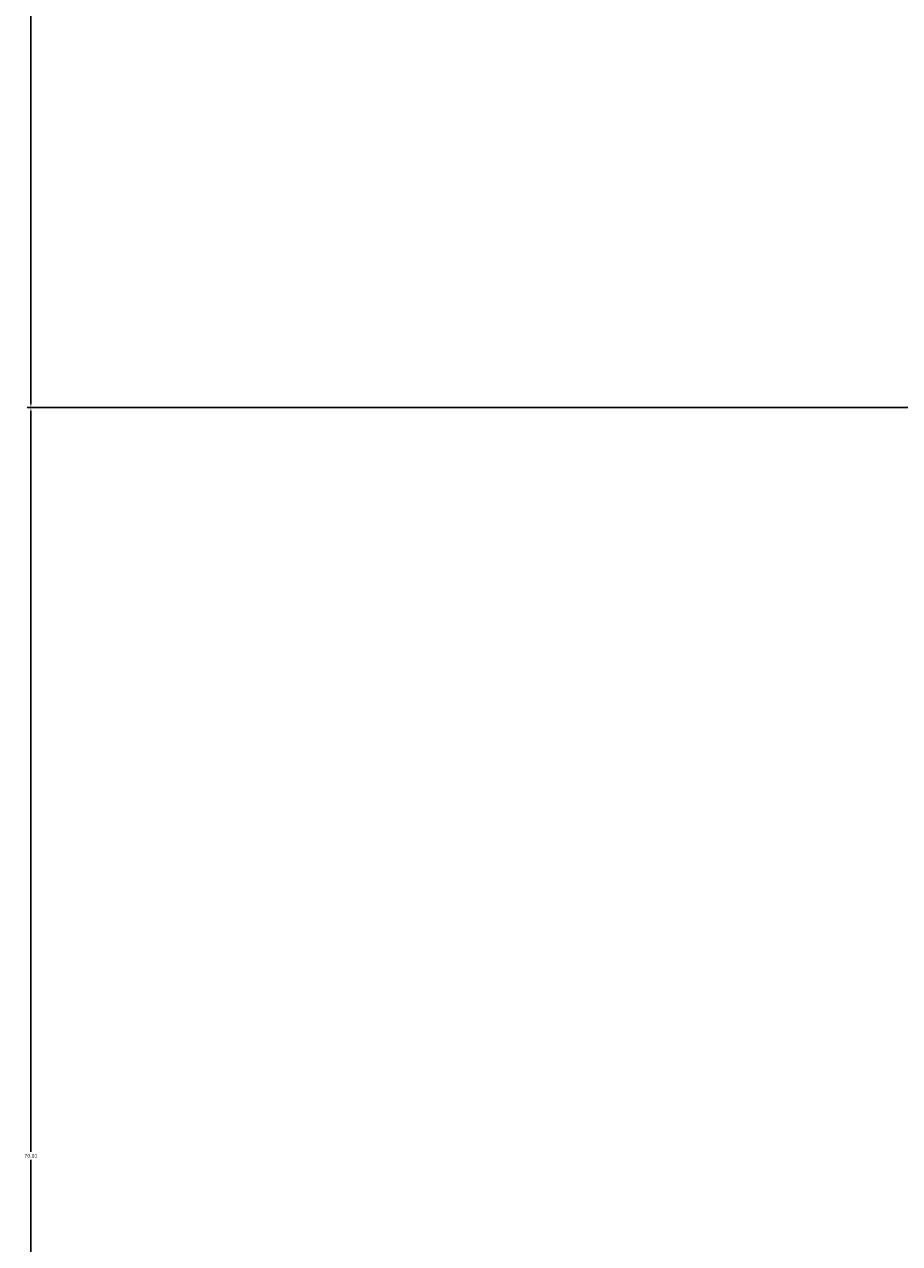
# Model space of a CAD drawing. Units: inches. Extents: x 738 to 1068, y 378 to 757.
# Tile 19 of 41: x 738 to 779, y 492 to 549. Entities that reach past the tile are written whole.
import ezdxf

# ---------------------------------------------------------------- set-up
doc = ezdxf.new("R2010")
doc.units = ezdxf.units.IN
doc.header["$MEASUREMENT"] = 0
doc.layers.add('A-ANNO-DIMS', color=2, linetype='Continuous', lineweight=18)
doc.styles.get("Standard").update_dxf_attribs({"font": 'arial.ttf'})
doc.dimstyles.get("Standard").update_dxf_attribs({"dimtxt": 0.18, "dimasz": 0.18, "dimexe": 0.18, "dimexo": 0.0625, "dimgap": 0.09, "dimtad": 0, "dimtih": 1, "dimtoh": 1, "dimdec": 4, "dimzin": 0, "dimdsep": 46, "dimtxsty": 'Standard', "dimcen": 0.09, "dimadec": 0, "dimazin": 0, "dimtfac": 1, "dimtdec": 4, "dimtofl": 0, "dimtmove": 0, "dimatfit": 3, "dimfxl": 1, "dimtolj": 1, "dimtzin": 0, "dimarcsym": 0})

# ---------------------------------------------------------------- blocks, each defined once
blk = doc.blocks.new('*D21')
at = {"layer": 'A-ANNO-DIMS', "color": 0, "lineweight": -2, "transparency": 16777216}
for p, q in [((781.427, 531.401), (738.194, 531.401)), ((738.374, 531.221), (738.374, 496.578)), ((738.374, 461.572), (738.374, 496.215)), ((781.427, 461.392), (738.194, 461.392))]:
    blk.add_line(p, q, dxfattribs=at)
at = {"layer": 'A-ANNO-DIMS', "color": 0, "transparency": 16777216}
for points in [[(738.344, 531.221), (738.404, 531.221), (738.374, 531.401)], [(738.344, 461.572), (738.404, 461.572), (738.374, 461.392)]]:
    blk.add_solid(points, dxfattribs=at)
at = {"layer": 'Defpoints', "color": 0, "transparency": 16777216}
for p in [(738.374, 531.401), (781.49, 531.401), (781.49, 461.392)]:
    blk.add_point(p, dxfattribs=at)
at = {"layer": 'A-ANNO-DIMS', "color": 0, "transparency": 16777216, "insert": (738.374, 496.396), "char_height": 0.18, "attachment_point": 5}
blk.add_mtext('\\A1;70.01', dxfattribs=at)
blk = doc.blocks.new('*D22')
at = {"layer": 'A-ANNO-DIMS', "color": 0, "lineweight": -2, "transparency": 16777216}
for p, q in [((781.422, 593.08), (738.194, 593.08)), ((738.374, 592.9), (738.374, 562.422)), ((738.374, 531.581), (738.374, 562.058)), ((781.427, 531.401), (738.194, 531.401))]:
    blk.add_line(p, q, dxfattribs=at)
at = {"layer": 'A-ANNO-DIMS', "color": 0, "transparency": 16777216}
for points in [[(738.344, 592.9), (738.404, 592.9), (738.374, 593.08)], [(738.344, 531.581), (738.404, 531.581), (738.374, 531.401)]]:
    blk.add_solid(points, dxfattribs=at)
at = {"layer": 'Defpoints', "color": 0, "transparency": 16777216}
for p in [(738.374, 593.08), (781.485, 593.08), (781.49, 531.401)]:
    blk.add_point(p, dxfattribs=at)
at = {"layer": 'A-ANNO-DIMS', "color": 0, "transparency": 16777216, "insert": (738.374, 562.24), "char_height": 0.18, "attachment_point": 5}
blk.add_mtext('\\A1;61.68', dxfattribs=at)

msp = doc.modelspace()

# ---------------------------------------------------------------- dimensions: what is measured, and where the dimension line sits
at = {"layer": 'A-ANNO-DIMS'}
for base, p1, p2, picture, middle in [((738.3736, 593.0796), (781.4897, 531.4009), (781.4846, 593.0796), '*D22', (738.3736, 562.2403)), ((738.3736, 531.4009), (781.4897, 461.3919), (781.4897, 531.4009), '*D21', (738.3736, 496.3964))]:
    dim = msp.add_linear_dim(base=base, p1=p1, p2=p2, angle=90, dimstyle='Standard', override={"dimdec": 2, "dimlfac": 1, "dimrnd": 0, "dimzin": 0, "dimdsep": 46, "dimlunit": 2}, dxfattribs=at)
    dim.commit()
    dim.dimension.update_dxf_attribs({"geometry": picture, "text_midpoint": middle})

doc.saveas('drawing.dxf')
